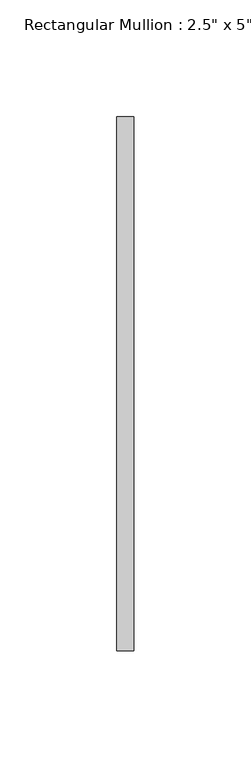
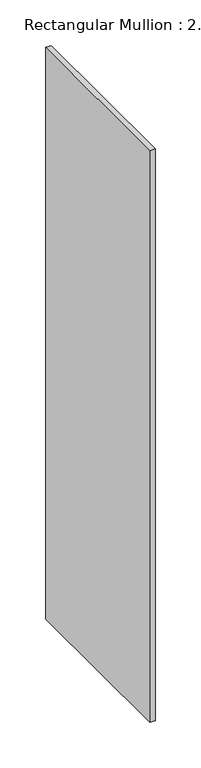
"""IFC4 building model written with IfcOpenShell, lengths in millimetres: member geometry."""

from ifc_helpers import new_model, si_unit, frame, origin, place, context, project, spatial, polyline, outline, extrude, source, transform, mapped, element, save


def member_d90fa784(model_context):
    return source(origin(), model_context, "Body", "SweptSolid", [
        extrude(outline(polyline([(0.0, 114.3), (0.0, -114.3), (-7.239, -114.3), (-7.239, 114.3), (0.0, 114.3)])), frame((0.0, 0.0, -767.0165), z_axis=(0.0, 0.0, 1.0), x_axis=(1.0, 0.0, 0.0)), (0.0, 0.0, 1.0), 767.0165),
    ])


if __name__ == "__main__":
    model = new_model("IFC4")
    model_context = context("Model", 3, world=origin())
    ifc_project = project(units=[si_unit("LENGTHUNIT", "METRE", prefix="MILLI")], contexts=[model_context])
    site = spatial("IfcSite", under=ifc_project)
    building = spatial("IfcBuilding", under=site)
    placement = place(None, origin())
    member_shape = member_d90fa784(model_context)
    element("IfcMember", 1, ObjectType="Rectangular Mullion : 2.5\" x 5\" rectangular", at=placement, inside=building, context=model_context, shape_type="MappedRepresentation", body=[
        mapped(member_shape, transform((0.0, 0.0, 0.0), x_axis=(1.0, 0.0, 0.0), y_axis=(0.0, 1.0, 0.0), z_axis=(0.0, 0.0, 1.0))),
    ])
    save(model, "model.ifc")

# Revit data of these elements
# Type "Rectangular Mullion : 2.5\" x 5\" rectangular"
#   built-in parameter 1007304 = 0.75 (stored number, unit not read)
#   built-in parameter 1007301 = 0.011875 (stored number, unit not read)
#   built-in parameter 1007300 = 0.011875 (stored number, unit not read)
# Element 1 (IfcMember, "Rectangular Mullion : 2.5\" x 5\" rectangular")
#   Materials on its faces: "WINDOW GLASS MATERIAL"
# Materials
#   "WINDOW GLASS MATERIAL": class "Generic", colour RGB 120 120 120, transparency 0, Cost = 0
